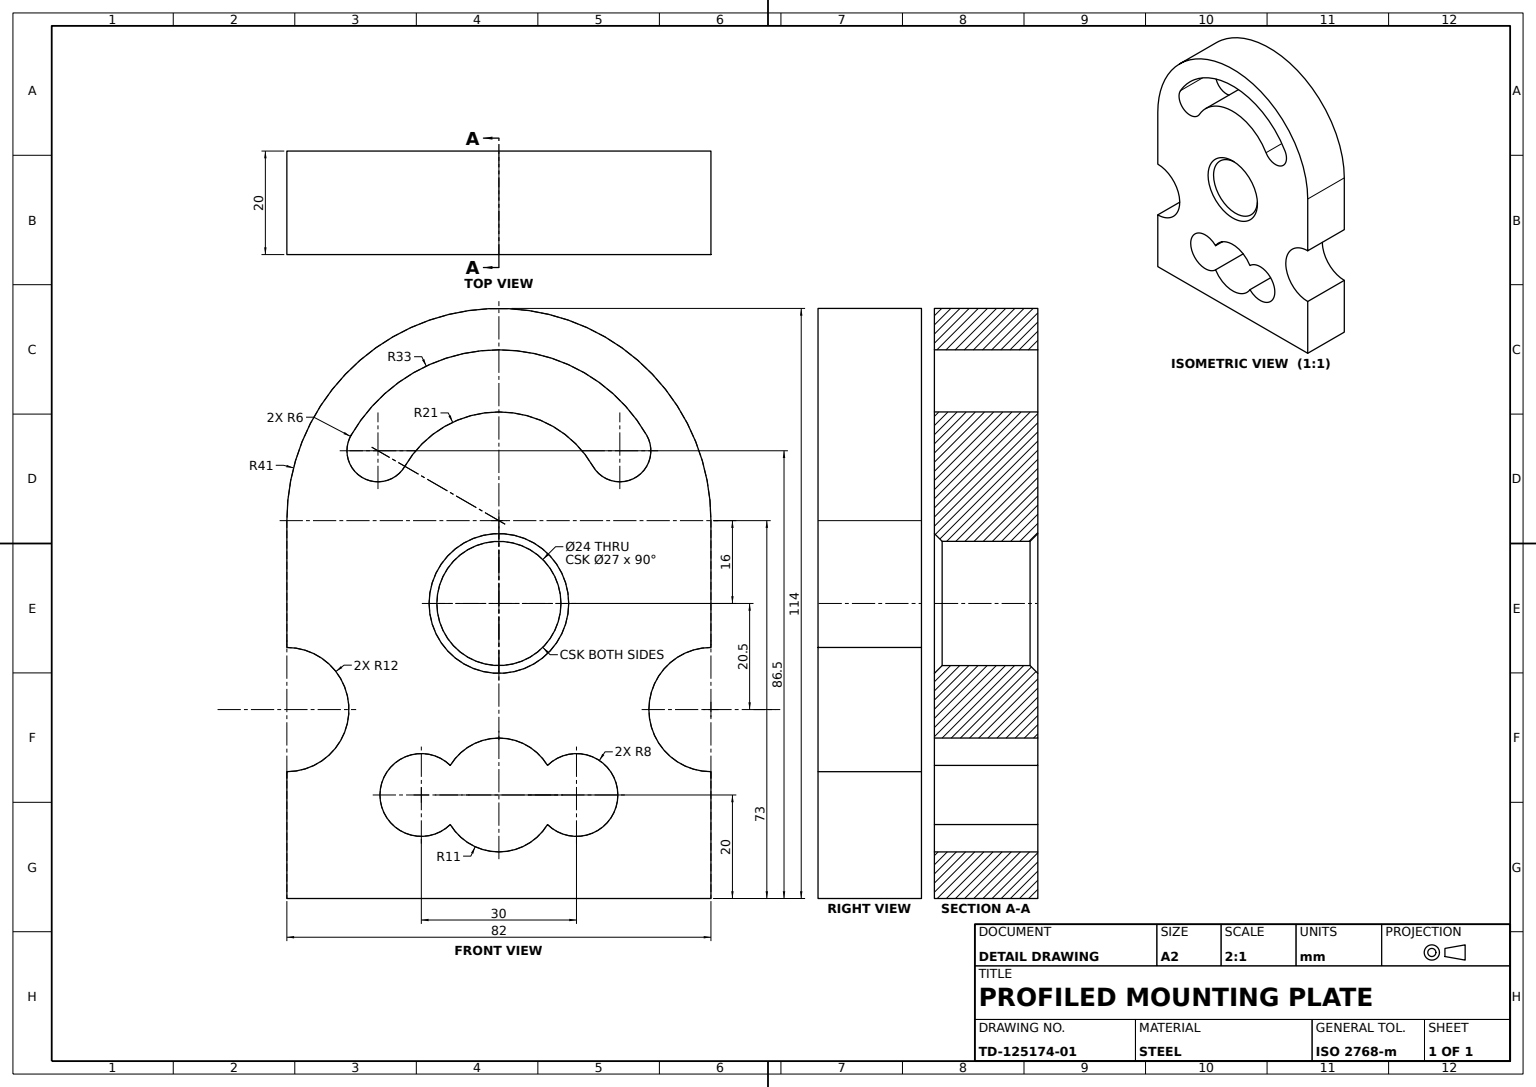
SolidWorks part; units mm, degrees
material "Plain Carbon Steel"
ref_plane "Front Plane" through (0, 0, 0) normal (0, 0, 1) x (1, 0, 0)
ref_plane "Top Plane" through (0, 0, 0) normal (0, 1, 0) x (1, 0, 0)
ref_plane "Right Plane" through (0, 0, 0) normal (1, 0, 0) x (0, 0, -1)
sketch "Plate Profile Sketch" plane through (0, 0, 0) normal (1, 0, 0) x (0, 0, -1)
  line L0 (0, 0) -> (0, 9) construction
  line L1 (0, 73) -> (25.1088, 73) construction
  line L2 (0, 73) -> (0, 169.0497) construction
  line L3 (0, 73) -> (-76.1773, 116.981) construction
  line L4 (0, 73) -> (76.1773, 116.981) construction
  line L5 (41, 73) -> (41, 48.5)
  line L6 (-41, 73) -> (-41, 48.5)
  line L7 (0, 0) -> (-41, 0)
  line L8 (0, 0) -> (41, 0)
  line L9 (-41, 24.5) -> (-41, 0)
  line L10 (41, 24.5) -> (41, 0)
  circle A1 centre (0, 57) radius 12
  arc A2 (9.4, 25.7131) -> (-9.4, 25.7131) centre (0, 20) ccw
  arc A3 (9.4, 14.2869) -> (9.4, 25.7131) centre (15, 20) ccw
  arc A4 (-9.4, 25.7131) -> (-9.4, 14.2869) centre (-15, 20) ccw
  arc A5 (-9.4, 14.2869) -> (9.4, 14.2869) centre (0, 20) ccw
  arc A6 (-23.3827, 86.5) -> (23.3827, 86.5) centre (0, 73) cw construction
  arc A7 (28.5788, 89.5) -> (-28.5788, 89.5) centre (0, 73) ccw
  arc A8 (18.1865, 83.5) -> (-18.1865, 83.5) centre (0, 73) ccw
  arc A9 (18.1865, 83.5) -> (28.5788, 89.5) centre (23.3827, 86.5) ccw
  arc A10 (-28.5788, 89.5) -> (-18.1865, 83.5) centre (-23.3827, 86.5) ccw
  arc A11 (41, 73) -> (-41, 73) centre (0, 73) ccw
  arc A12 (41, 48.5) -> (41, 24.5) centre (41, 36.5) ccw
  arc A13 (-41, 24.5) -> (-41, 48.5) centre (-41, 36.5) ccw
  point P19 (0, 100)
  dimension "D1" = 57
  dimension "D2" = 24
  dimension "D4" = 22
  dimension "D7" = 16
  dimension "D8" = 16
  dimension "D12" = 27
  dimension "D13" = 6
  dimension "D14" = 82
  dimension "D17" = 24
  dimension "D18" = 24
  dimension "D3" = 20
  dimension "D5" = 30
  dimension "D6" = 15
  dimension "D9" = 15
  dimension "D10" = 73
  dimension "D11" = 60
  dimension "D15" = 36.5
  dimension "D16" = 36.5
extrude "Profiled Plate 20mm" add sketch "Plate Profile Sketch" along normal blind 20
chamfer "Bore Chamfer 1.5x45deg" distance 1.5 angle 45 2 edges at (0, 57, -12) (20, 57, -12)
